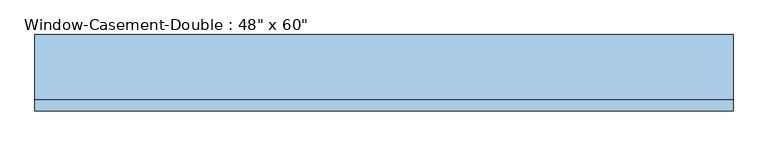
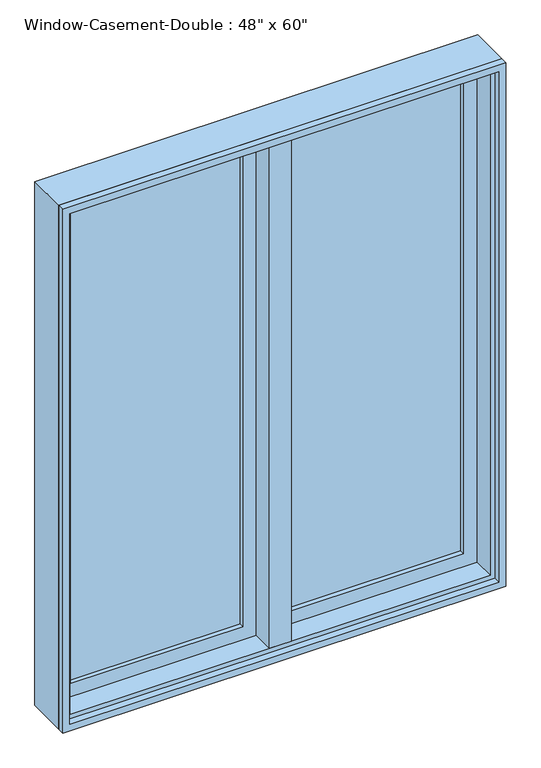
"""IFC4 building model written with IfcOpenShell, lengths in millimetres: window geometry."""

from ifc_helpers import new_model, si_unit, frame, origin, place, context, project, spatial, polyline, outline, extrude, faceted_brep, source, transform, mapped, element, save


def window_d9d3dda5(model_context):
    return source(origin(), model_context, "Body", "SolidModel", [
        faceted_brep([(9.525, 76.2, 2425.7), (-9.525, 76.2, 2425.7), (-9.525, 25.4, 2425.7), (9.525, 25.4, 2425.7), (9.525, 76.2, 927.1), (9.525, 25.4, 927.1), (-9.525, 25.4, 927.1), (-9.525, 76.2, 927.1), (-9.525, 25.4, 946.15), (-9.525, 25.4, 2406.65), (-30.1625, 25.4, 946.15), (-30.1625, 25.4, 2406.65), (-30.1625, -38.1, 946.15), (-30.1625, -38.1, 2406.65), (30.1625, -38.1, 946.15), (30.1625, -38.1, 2406.65), (30.1625, 25.4, 946.15), (30.1625, 25.4, 2406.65), (9.525, 25.4, 946.15), (9.525, 25.4, 2406.65)], [[[0, 1, 2, 3]], [[4, 5, 6, 7]], [[1, 0, 4, 7]], [[2, 1, 7, 6, 8, 9]], [[9, 8, 10, 11]], [[11, 10, 12, 13]], [[13, 12, 14, 15]], [[15, 14, 16, 17]], [[17, 16, 18, 19]], [[0, 3, 19, 18, 5, 4]], [[18, 8, 6, 5]], [[9, 19, 3, 2]], [[8, 18, 16, 14, 12, 10]], [[19, 9, 11, 13, 15, 17]]]),
        extrude(outline(polyline([(-66.675, 57.15), (-66.675, 50.8), (-539.75, 50.8), (-539.75, 57.15), (-66.675, 57.15)])), frame((0.0, 0.0, 984.25), z_axis=(0.0, 0.0, 1.0), x_axis=(1.0, 0.0, 0.0)), (0.0, 0.0, 1.0), 1384.3),
        extrude(outline(polyline([(-539.75, 38.1), (-539.75, 44.45), (-66.675, 44.45), (-66.675, 38.1), (-539.75, 38.1)])), frame((0.0, 0.0, 984.25), z_axis=(0.0, 0.0, 1.0), x_axis=(1.0, 0.0, 0.0)), (0.0, 0.0, 1.0), 1384.3),
        extrude(outline(polyline([(539.75, 57.15), (539.75, 50.8), (66.675, 50.8), (66.675, 57.15), (539.75, 57.15)])), frame((0.0, 0.0, 984.25), z_axis=(0.0, 0.0, 1.0), x_axis=(1.0, 0.0, 0.0)), (0.0, 0.0, 1.0), 1384.3),
        extrude(outline(polyline([(66.675, 38.1), (66.675, 44.45), (539.75, 44.45), (539.75, 38.1), (66.675, 38.1)])), frame((0.0, 0.0, 984.25), z_axis=(0.0, 0.0, 1.0), x_axis=(1.0, 0.0, 0.0)), (0.0, 0.0, 1.0), 1384.3),
        extrude(outline(polyline([(2425.7, -596.9), (927.1, -596.9), (927.1, -9.525), (2425.7, -9.525), (2425.7, -596.9)]), holes=[polyline([(2368.55, -66.675), (984.25, -66.675), (984.25, -539.75), (2368.55, -539.75), (2368.55, -66.675)])]), frame((0.0, 25.4, 0.0), z_axis=(0.0, 1.0, 0.0), x_axis=(0.0, 0.0, 1.0)), (0.0, 0.0, 1.0), 44.45),
        extrude(outline(polyline([(927.1, 596.9), (2425.7, 596.9), (2425.7, 9.525), (927.1, 9.525), (927.1, 596.9)]), holes=[polyline([(984.25, 66.675), (2368.55, 66.675), (2368.55, 539.75), (984.25, 539.75), (984.25, 66.675)])]), frame((0.0, 25.4, 0.0), z_axis=(0.0, 1.0, 0.0), x_axis=(0.0, 0.0, 1.0)), (0.0, 0.0, 1.0), 44.45),
        extrude(outline(polyline([(2438.4, -609.6), (914.4, -609.6), (914.4, 609.6), (2438.4, 609.6), (2438.4, -609.6)]), holes=[polyline([(2419.35, 590.55), (933.45, 590.55), (933.45, -590.55), (2419.35, -590.55), (2419.35, 590.55)])]), frame((0.0, -57.15, 0.0), z_axis=(0.0, 1.0, 0.0), x_axis=(0.0, 0.0, 1.0)), (0.0, 0.0, 1.0), 19.05),
        faceted_brep([(577.85, 25.4, 2406.65), (577.85, -38.1, 2406.65), (-577.85, -38.1, 2406.65), (-577.85, 25.4, 2406.65), (596.9, 76.2, 2425.7), (596.9, 25.4, 2425.7), (-596.9, 25.4, 2425.7), (-596.9, 76.2, 2425.7), (609.6, -38.1, 2438.4), (609.6, 76.2, 2438.4), (-609.6, 76.2, 2438.4), (-609.6, -38.1, 2438.4), (-577.85, -38.1, 946.15), (-577.85, 25.4, 946.15), (-596.9, 25.4, 927.1), (-596.9, 76.2, 927.1), (-609.6, 76.2, 914.4), (-609.6, -38.1, 914.4), (577.85, -38.1, 946.15), (577.85, 25.4, 946.15), (596.9, 25.4, 927.1), (596.9, 76.2, 927.1), (609.6, 76.2, 914.4), (609.6, -38.1, 914.4)], [[[0, 1, 2, 3]], [[4, 5, 6, 7]], [[8, 9, 10, 11]], [[3, 2, 12, 13]], [[7, 6, 14, 15]], [[11, 10, 16, 17]], [[13, 12, 18, 19]], [[15, 14, 20, 21]], [[17, 16, 22, 23]], [[11, 17, 23, 8], [1, 18, 12, 2]], [[19, 18, 1, 0]], [[5, 20, 14, 6], [3, 13, 19, 0]], [[21, 20, 5, 4]], [[23, 22, 9, 8]], [[9, 22, 16, 10], [7, 15, 21, 4]]]),
    ])


if __name__ == "__main__":
    model = new_model("IFC4")
    model_context = context("Model", 3, world=origin())
    ifc_project = project(units=[si_unit("LENGTHUNIT", "METRE", prefix="MILLI")], contexts=[model_context])
    site = spatial("IfcSite", under=ifc_project)
    building = spatial("IfcBuilding", under=site)
    placement = place(None, origin())
    window_shape = window_d9d3dda5(model_context)
    element("IfcWindow", 1, ObjectType="Window-Casement-Double : 48\" x 60\"", at=placement, inside=building, context=model_context, shape_type="MappedRepresentation", body=[
        mapped(window_shape, transform((0.0, 0.0, 0.0), x_axis=(1.0, 0.0, 0.0), y_axis=(0.0, 1.0, 0.0), z_axis=(0.0, 0.0, 1.0))),
    ])
    save(model, "model.ifc")

# Revit data of these elements
# Type "Window-Casement-Double : 48\" x 60\""
#   Type Mark = "16"
#   Fire Rating = "0.5h"
#   Assembly Code = "B2020100"
#   Analytic Construction = "Double glazing - domestic"
#   Frame Extension [instance default] = 0' - 0 1/4"
#   Window Inset [instance default] = 0' - 0"
#   Wall Thickness [instance default] = 0' - 6"
#   Interior Wall Closure [instance default] = 0' - 2 1/4"
#   Half Width = 2' - 0"
#   Visual Light Transmittance = 0.81
#   Thermal Resistance (R) = 1.8146 (h·ft²·°F)/BTU
#   Solar Heat Gain Coefficient = 0.76
#   Rough Width = 4' - 0 1/2"
#   Rough Height = 5' - 0 1/2"
#   Height = 5' - 0"
#   Heat Transfer Coefficient (U) = 0.5511 BTU/(h·ft²·°F)
#   Exterior Wall Closure [instance default] = 0' - 1 1/4"
#   Extension Jamb [instance default] = 0' - 2 1/4"
#   Default Sill Height = 3' - 0"
#   Width = 4' - 0"
#   Define Thermal Properties by = 0
#   Muntin Visibility = yes
#   Interior Trim Visibility [instance default] = yes
#   Exterior Trim Visibility [instance default] = yes
#   Extension Jamb Visibility [instance default] = yes
#   Interior Trim Material = Wood - Stained
#   Muntin Pattern = Muntin Pattern_2x2 : Muntin Pattern_2x2
#   Interior Trim = Trim-Window-Interior-Flat : Picture Frame
#   Interior Frame Material = Wood - Stained
#   Glass Panel Material = Glass
#   Exterior Trim Material = Clad - White
#   Exterior Trim = Trim-Window-Exterior-Flat : with Sill
#   Exterior Frame Material = Clad - White
#   Wall Closure = (empty or 0)
# Element 1 (IfcWindow, "Window-Casement-Double : 48\" x 60\"")
#   Wall Thickness = 0' - 4 1/2"
#   Extension Jamb = 0' - 0 3/4"
#   Materials on its faces: "Wood - Stained", "Glass", "Clad - White"
# Materials
#   "Wood - Stained": class "Wood", colour RGB 224 178 126, transparency 0, Cost = 0
#   "Glass": class "Glass", colour RGB 0 128 192, transparency 0.75, Description = "Soda Lime Glass", Cost = 0
#   "Clad - White": class "Wood", colour RGB 242 242 238, transparency 0, Cost = 0
